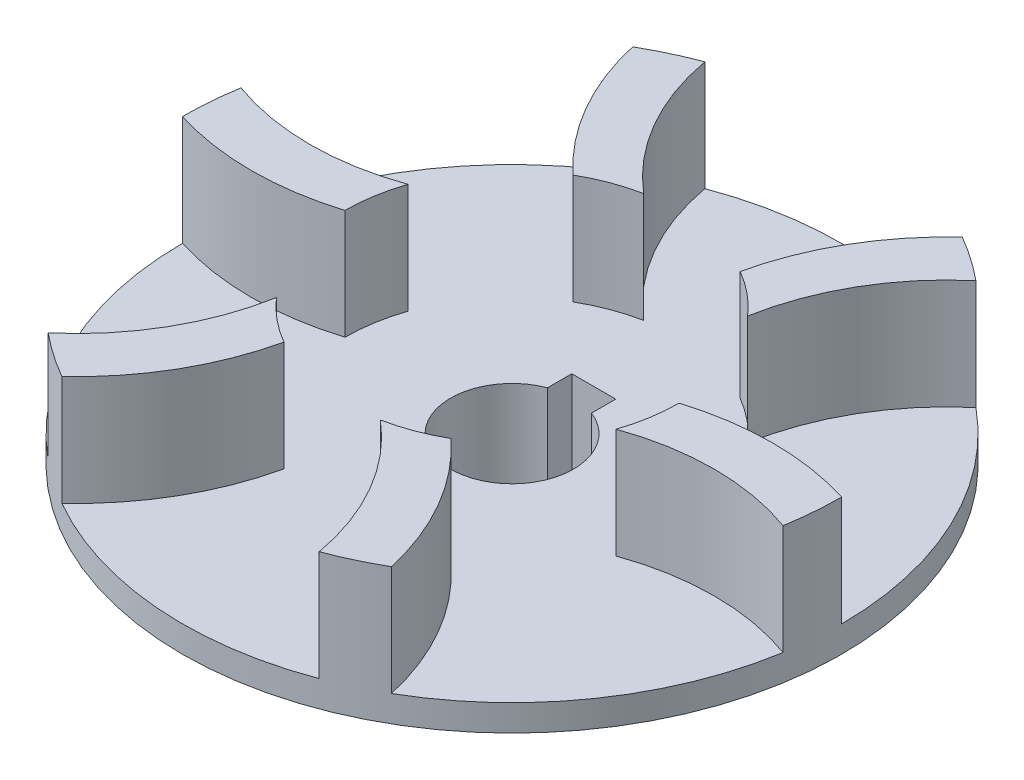
ISO-10303-21;
HEADER;
FILE_DESCRIPTION(('STEP AP214'),'2;1');
FILE_NAME('part.step','',(''),(''),'','','');
FILE_SCHEMA(('AUTOMOTIVE_DESIGN { 1 0 10303 214 1 1 1 1 }'));
ENDSEC;
DATA;
#1=APPLICATION_CONTEXT('core data for automotive mechanical design processes');
#2=APPLICATION_PROTOCOL_DEFINITION('international standard','automotive_design',2000,#1);
#3=PRODUCT_CONTEXT('',#1,'mechanical');
#4=PRODUCT('Part','Part','',(#3));
#5=PRODUCT_RELATED_PRODUCT_CATEGORY('part','',(#4));
#6=PRODUCT_DEFINITION_FORMATION('','',#4);
#7=PRODUCT_DEFINITION_CONTEXT('part definition',#1,'design');
#8=PRODUCT_DEFINITION('design','',#6,#7);
#9=PRODUCT_DEFINITION_SHAPE('','',#8);
#10=(LENGTH_UNIT() NAMED_UNIT(*) SI_UNIT(.MILLI.,.METRE.));
#11=(NAMED_UNIT(*) PLANE_ANGLE_UNIT() SI_UNIT($,.RADIAN.));
#12=(NAMED_UNIT(*) SI_UNIT($,.STERADIAN.) SOLID_ANGLE_UNIT());
#13=UNCERTAINTY_MEASURE_WITH_UNIT(LENGTH_MEASURE(1.E-05),#10,'distance_accuracy_value','');
#14=(GEOMETRIC_REPRESENTATION_CONTEXT(3) GLOBAL_UNCERTAINTY_ASSIGNED_CONTEXT((#13)) GLOBAL_UNIT_ASSIGNED_CONTEXT((#10,
#11,#12)) REPRESENTATION_CONTEXT('',''));
#15=CARTESIAN_POINT('',(0.,0.,0.));
#16=DIRECTION('',(0.,0.,1.));
#17=DIRECTION('',(1.,0.,0.));
#18=AXIS2_PLACEMENT_3D('',#15,#16,#17);
#19=CARTESIAN_POINT('',(0.,1.5,0.));
#20=DIRECTION('',(0.,-1.,0.));
#21=DIRECTION('',(0.,0.,-1.));
#22=AXIS2_PLACEMENT_3D('',#19,#20,#21);
#23=CYLINDRICAL_SURFACE('',#22,7.);
#24=DIRECTION('',(0.,-1.,0.));
#25=VECTOR('',#24,1.);
#26=CARTESIAN_POINT('',(2.5,1.5,-6.53834841531101));
#27=LINE('',#26,#25);
#28=CARTESIAN_POINT('',(2.5,1.5,-6.53834841531101));
#29=VERTEX_POINT('',#28);
#30=CARTESIAN_POINT('',(2.5,-17.5,-6.53834841531101));
#31=VERTEX_POINT('',#30);
#32=EDGE_CURVE('E238',#29,#31,#27,.T.);
#33=ORIENTED_EDGE('',*,*,#32,.T.);
#34=CARTESIAN_POINT('',(0.,-17.5,0.));
#35=DIRECTION('',(0.,-1.,0.));
#36=DIRECTION('',(0.,0.,-1.));
#37=AXIS2_PLACEMENT_3D('',#34,#35,#36);
#38=CIRCLE('',#37,7.);
#39=CARTESIAN_POINT('',(-2.5,-17.5,-6.53834841531101));
#40=VERTEX_POINT('',#39);
#41=EDGE_CURVE('E236',#40,#31,#38,.F.);
#42=ORIENTED_EDGE('',*,*,#41,.F.);
#43=DIRECTION('',(0.,-1.,0.));
#44=VECTOR('',#43,1.);
#45=CARTESIAN_POINT('',(-2.5,1.5,-6.53834841531101));
#46=LINE('',#45,#44);
#47=CARTESIAN_POINT('',(-2.5,1.5,-6.53834841531101));
#48=VERTEX_POINT('',#47);
#49=EDGE_CURVE('E221',#48,#40,#46,.T.);
#50=ORIENTED_EDGE('',*,*,#49,.F.);
#51=CARTESIAN_POINT('',(0.,1.5,0.));
#52=DIRECTION('',(0.,1.,0.));
#53=DIRECTION('',(0.,0.,1.));
#54=AXIS2_PLACEMENT_3D('',#51,#52,#53);
#55=CIRCLE('',#54,7.);
#56=EDGE_CURVE('E400',#48,#29,#55,.T.);
#57=ORIENTED_EDGE('',*,*,#56,.T.);
#58=EDGE_LOOP('',(#33,#42,#50,#57));
#59=FACE_BOUND('',#58,.T.);
#60=ADVANCED_FACE('F41',(#59),#23,.F.);
#61=CARTESIAN_POINT('',(-2.5,1.5,0.));
#62=DIRECTION('',(1.,0.,0.));
#63=DIRECTION('',(0.,0.,-1.));
#64=AXIS2_PLACEMENT_3D('',#61,#62,#63);
#65=PLANE('',#64);
#66=ORIENTED_EDGE('',*,*,#49,.T.);
#67=DIRECTION('',(0.,0.,1.));
#68=VECTOR('',#67,1.);
#69=CARTESIAN_POINT('',(-2.5,-17.5,0.));
#70=LINE('',#69,#68);
#71=CARTESIAN_POINT('',(-2.5,-17.5,-9.3));
#72=VERTEX_POINT('',#71);
#73=EDGE_CURVE('E230',#72,#40,#70,.T.);
#74=ORIENTED_EDGE('',*,*,#73,.F.);
#75=DIRECTION('',(0.,-1.,0.));
#76=VECTOR('',#75,1.);
#77=CARTESIAN_POINT('',(-2.5,1.5,-9.3));
#78=LINE('',#77,#76);
#79=CARTESIAN_POINT('',(-2.5,1.5,-9.3));
#80=VERTEX_POINT('',#79);
#81=EDGE_CURVE('E234',#80,#72,#78,.T.);
#82=ORIENTED_EDGE('',*,*,#81,.F.);
#83=DIRECTION('',(0.,0.,1.));
#84=VECTOR('',#83,1.);
#85=CARTESIAN_POINT('',(-2.5,1.5,0.));
#86=LINE('',#85,#84);
#87=EDGE_CURVE('E228',#80,#48,#86,.T.);
#88=ORIENTED_EDGE('',*,*,#87,.T.);
#89=EDGE_LOOP('',(#66,#74,#82,#88));
#90=FACE_BOUND('',#89,.T.);
#91=ADVANCED_FACE('F227',(#90),#65,.T.);
#92=CARTESIAN_POINT('',(0.,1.5,-9.3));
#93=DIRECTION('',(0.,0.,1.));
#94=DIRECTION('',(1.,0.,0.));
#95=AXIS2_PLACEMENT_3D('',#92,#93,#94);
#96=PLANE('',#95);
#97=ORIENTED_EDGE('',*,*,#81,.T.);
#98=DIRECTION('',(-1.,0.,0.));
#99=VECTOR('',#98,1.);
#100=CARTESIAN_POINT('',(0.,-17.5,-9.3));
#101=LINE('',#100,#99);
#102=CARTESIAN_POINT('',(2.5,-17.5,-9.3));
#103=VERTEX_POINT('',#102);
#104=EDGE_CURVE('E249',#103,#72,#101,.T.);
#105=ORIENTED_EDGE('',*,*,#104,.F.);
#106=DIRECTION('',(0.,-1.,0.));
#107=VECTOR('',#106,1.);
#108=CARTESIAN_POINT('',(2.5,1.5,-9.3));
#109=LINE('',#108,#107);
#110=CARTESIAN_POINT('',(2.5,1.5,-9.3));
#111=VERTEX_POINT('',#110);
#112=EDGE_CURVE('E415',#111,#103,#109,.T.);
#113=ORIENTED_EDGE('',*,*,#112,.F.);
#114=DIRECTION('',(-1.,0.,0.));
#115=VECTOR('',#114,1.);
#116=CARTESIAN_POINT('',(0.,1.5,-9.3));
#117=LINE('',#116,#115);
#118=EDGE_CURVE('E399',#111,#80,#117,.T.);
#119=ORIENTED_EDGE('',*,*,#118,.T.);
#120=EDGE_LOOP('',(#97,#105,#113,#119));
#121=FACE_BOUND('',#120,.T.);
#122=ADVANCED_FACE('F513',(#121),#96,.T.);
#123=CARTESIAN_POINT('',(2.5,1.5,0.));
#124=DIRECTION('',(1.,0.,0.));
#125=DIRECTION('',(0.,0.,-1.));
#126=AXIS2_PLACEMENT_3D('',#123,#124,#125);
#127=PLANE('',#126);
#128=ORIENTED_EDGE('',*,*,#112,.T.);
#129=DIRECTION('',(0.,0.,-1.));
#130=VECTOR('',#129,1.);
#131=CARTESIAN_POINT('',(2.5,-17.5,0.));
#132=LINE('',#131,#130);
#133=EDGE_CURVE('E241',#31,#103,#132,.T.);
#134=ORIENTED_EDGE('',*,*,#133,.F.);
#135=ORIENTED_EDGE('',*,*,#32,.F.);
#136=DIRECTION('',(0.,0.,1.));
#137=VECTOR('',#136,1.);
#138=CARTESIAN_POINT('',(2.5,1.5,0.));
#139=LINE('',#138,#137);
#140=EDGE_CURVE('E401',#111,#29,#139,.T.);
#141=ORIENTED_EDGE('',*,*,#140,.F.);
#142=EDGE_LOOP('',(#128,#134,#135,#141));
#143=FACE_BOUND('',#142,.T.);
#144=ADVANCED_FACE('F518',(#143),#127,.F.);
#145=CARTESIAN_POINT('',(0.,1.5,0.));
#146=DIRECTION('',(0.,-1.,0.));
#147=DIRECTION('',(0.,0.,-1.));
#148=AXIS2_PLACEMENT_3D('',#145,#146,#147);
#149=CYLINDRICAL_SURFACE('',#148,37.5);
#150=CARTESIAN_POINT('',(0.,1.5,0.));
#151=DIRECTION('',(0.,1.,0.));
#152=DIRECTION('',(0.,0.,1.));
#153=AXIS2_PLACEMENT_3D('',#150,#151,#152);
#154=CIRCLE('',#153,37.5);
#155=CARTESIAN_POINT('',(18.7500000000004,1.5,-32.4759526419162));
#156=VERTEX_POINT('',#155);
#157=CARTESIAN_POINT('',(-13.1678223706898,1.5,-35.1120841593597));
#158=VERTEX_POINT('',#157);
#159=EDGE_CURVE('E410',#156,#158,#154,.T.);
#160=ORIENTED_EDGE('',*,*,#159,.F.);
#161=DIRECTION('',(0.,-1.,0.));
#162=VECTOR('',#161,1.);
#163=CARTESIAN_POINT('',(18.7500000000004,14.,-32.4759526419162));
#164=LINE('',#163,#162);
#165=CARTESIAN_POINT('',(18.7500000000004,14.,-32.4759526419162));
#166=VERTEX_POINT('',#165);
#167=EDGE_CURVE('E261',#166,#156,#164,.T.);
#168=ORIENTED_EDGE('',*,*,#167,.F.);
#169=CARTESIAN_POINT('',(0.,14.,0.));
#170=DIRECTION('',(0.,1.,0.));
#171=DIRECTION('',(0.,0.,1.));
#172=AXIS2_PLACEMENT_3D('',#169,#170,#171);
#173=CIRCLE('',#172,37.5);
#174=CARTESIAN_POINT('',(23.8240456764779,14.,-28.9597107652182));
#175=VERTEX_POINT('',#174);
#176=EDGE_CURVE('E277',#175,#166,#173,.T.);
#177=ORIENTED_EDGE('',*,*,#176,.F.);
#178=DIRECTION('',(0.,-1.,0.));
#179=VECTOR('',#178,1.);
#180=CARTESIAN_POINT('',(23.8240456764779,14.,-28.9597107652182));
#181=LINE('',#180,#179);
#182=CARTESIAN_POINT('',(23.8240456764779,1.5,-28.9597107652182));
#183=VERTEX_POINT('',#182);
#184=EDGE_CURVE('E256',#175,#183,#181,.T.);
#185=ORIENTED_EDGE('',*,*,#184,.T.);
#186=CARTESIAN_POINT('',(37.5,1.5,0.));
#187=VERTEX_POINT('',#186);
#188=EDGE_CURVE('E407',#187,#183,#154,.T.);
#189=ORIENTED_EDGE('',*,*,#188,.F.);
#190=DIRECTION('',(0.,-1.,0.));
#191=VECTOR('',#190,1.);
#192=CARTESIAN_POINT('',(37.5,14.,0.));
#193=LINE('',#192,#191);
#194=CARTESIAN_POINT('',(37.5,14.,0.));
#195=VERTEX_POINT('',#194);
#196=EDGE_CURVE('E388',#195,#187,#193,.T.);
#197=ORIENTED_EDGE('',*,*,#196,.F.);
#198=CARTESIAN_POINT('',(0.,14.,0.));
#199=DIRECTION('',(0.,1.,0.));
#200=DIRECTION('',(0.,0.,1.));
#201=AXIS2_PLACEMENT_3D('',#198,#199,#200);
#202=CIRCLE('',#201,37.5);
#203=CARTESIAN_POINT('',(36.9918680471677,14.,6.15237339414113));
#204=VERTEX_POINT('',#203);
#205=EDGE_CURVE('E376',#204,#195,#202,.T.);
#206=ORIENTED_EDGE('',*,*,#205,.F.);
#207=DIRECTION('',(0.,-1.,0.));
#208=VECTOR('',#207,1.);
#209=CARTESIAN_POINT('',(36.9918680471677,14.,6.15237339414113));
#210=LINE('',#209,#208);
#211=CARTESIAN_POINT('',(36.9918680471677,1.5,6.15237339414113));
#212=VERTEX_POINT('',#211);
#213=EDGE_CURVE('E395',#204,#212,#210,.T.);
#214=ORIENTED_EDGE('',*,*,#213,.T.);
#215=CARTESIAN_POINT('',(18.7499999999999,1.5,32.4759526419165));
#216=VERTEX_POINT('',#215);
#217=EDGE_CURVE('E403',#216,#212,#154,.T.);
#218=ORIENTED_EDGE('',*,*,#217,.F.);
#219=DIRECTION('',(0.,-1.,0.));
#220=VECTOR('',#219,1.);
#221=CARTESIAN_POINT('',(18.7499999999999,14.,32.4759526419165));
#222=LINE('',#221,#220);
#223=CARTESIAN_POINT('',(18.7499999999999,14.,32.4759526419165));
#224=VERTEX_POINT('',#223);
#225=EDGE_CURVE('E355',#224,#216,#222,.T.);
#226=ORIENTED_EDGE('',*,*,#225,.F.);
#227=CARTESIAN_POINT('',(0.,14.,0.));
#228=DIRECTION('',(0.,1.,0.));
#229=DIRECTION('',(0.,0.,1.));
#230=AXIS2_PLACEMENT_3D('',#227,#228,#229);
#231=CIRCLE('',#230,37.5);
#232=CARTESIAN_POINT('',(13.16782237069,14.,35.1120841593597));
#233=VERTEX_POINT('',#232);
#234=EDGE_CURVE('E366',#233,#224,#231,.T.);
#235=ORIENTED_EDGE('',*,*,#234,.F.);
#236=DIRECTION('',(0.,-1.,0.));
#237=VECTOR('',#236,1.);
#238=CARTESIAN_POINT('',(13.16782237069,14.,35.1120841593597));
#239=LINE('',#238,#237);
#240=CARTESIAN_POINT('',(13.16782237069,1.5,35.1120841593597));
#241=VERTEX_POINT('',#240);
#242=EDGE_CURVE('E348',#233,#241,#239,.T.);
#243=ORIENTED_EDGE('',*,*,#242,.T.);
#244=CARTESIAN_POINT('',(-18.7500000000001,1.5,32.4759526419164));
#245=VERTEX_POINT('',#244);
#246=EDGE_CURVE('E477',#245,#241,#154,.T.);
#247=ORIENTED_EDGE('',*,*,#246,.F.);
#248=DIRECTION('',(0.,-1.,0.));
#249=VECTOR('',#248,1.);
#250=CARTESIAN_POINT('',(-18.7500000000002,14.,32.4759526419164));
#251=LINE('',#250,#249);
#252=CARTESIAN_POINT('',(-18.7500000000002,14.,32.4759526419164));
#253=VERTEX_POINT('',#252);
#254=EDGE_CURVE('E329',#253,#245,#251,.T.);
#255=ORIENTED_EDGE('',*,*,#254,.F.);
#256=CARTESIAN_POINT('',(0.,14.,0.));
#257=DIRECTION('',(0.,1.,0.));
#258=DIRECTION('',(0.,0.,1.));
#259=AXIS2_PLACEMENT_3D('',#256,#257,#258);
#260=CIRCLE('',#259,37.5);
#261=CARTESIAN_POINT('',(-23.8240456764777,14.,28.9597107652184));
#262=VERTEX_POINT('',#261);
#263=EDGE_CURVE('E344',#262,#253,#260,.T.);
#264=ORIENTED_EDGE('',*,*,#263,.F.);
#265=DIRECTION('',(0.,-1.,0.));
#266=VECTOR('',#265,1.);
#267=CARTESIAN_POINT('',(-23.8240456764777,14.,28.9597107652184));
#268=LINE('',#267,#266);
#269=CARTESIAN_POINT('',(-23.8240456764777,1.5,28.9597107652184));
#270=VERTEX_POINT('',#269);
#271=EDGE_CURVE('E330',#262,#270,#268,.T.);
#272=ORIENTED_EDGE('',*,*,#271,.T.);
#273=CARTESIAN_POINT('',(-37.5,1.5,-2.63677968348475E-13));
#274=VERTEX_POINT('',#273);
#275=EDGE_CURVE('E480',#274,#270,#154,.T.);
#276=ORIENTED_EDGE('',*,*,#275,.F.);
#277=DIRECTION('',(0.,-1.,0.));
#278=VECTOR('',#277,1.);
#279=CARTESIAN_POINT('',(-37.5,14.,-2.63677968348475E-13));
#280=LINE('',#279,#278);
#281=CARTESIAN_POINT('',(-37.5,14.,-2.63677968348475E-13));
#282=VERTEX_POINT('',#281);
#283=EDGE_CURVE('E307',#282,#274,#280,.T.);
#284=ORIENTED_EDGE('',*,*,#283,.F.);
#285=CARTESIAN_POINT('',(0.,14.,0.));
#286=DIRECTION('',(0.,1.,0.));
#287=DIRECTION('',(0.,0.,1.));
#288=AXIS2_PLACEMENT_3D('',#285,#286,#287);
#289=CIRCLE('',#288,37.5);
#290=CARTESIAN_POINT('',(-36.9918680471676,14.,-6.15237339414141));
#291=VERTEX_POINT('',#290);
#292=EDGE_CURVE('E325',#291,#282,#289,.T.);
#293=ORIENTED_EDGE('',*,*,#292,.F.);
#294=DIRECTION('',(0.,-1.,0.));
#295=VECTOR('',#294,1.);
#296=CARTESIAN_POINT('',(-36.9918680471676,14.,-6.15237339414141));
#297=LINE('',#296,#295);
#298=CARTESIAN_POINT('',(-36.9918680471676,1.5,-6.15237339414141));
#299=VERTEX_POINT('',#298);
#300=EDGE_CURVE('E302',#291,#299,#297,.T.);
#301=ORIENTED_EDGE('',*,*,#300,.T.);
#302=CARTESIAN_POINT('',(-18.7499999999997,1.5,-32.4759526419166));
#303=VERTEX_POINT('',#302);
#304=EDGE_CURVE('E478',#303,#299,#154,.T.);
#305=ORIENTED_EDGE('',*,*,#304,.F.);
#306=DIRECTION('',(0.,-1.,0.));
#307=VECTOR('',#306,1.);
#308=CARTESIAN_POINT('',(-18.7499999999997,14.,-32.4759526419166));
#309=LINE('',#308,#307);
#310=CARTESIAN_POINT('',(-18.7499999999997,14.,-32.4759526419166));
#311=VERTEX_POINT('',#310);
#312=EDGE_CURVE('E281',#311,#303,#309,.T.);
#313=ORIENTED_EDGE('',*,*,#312,.F.);
#314=CARTESIAN_POINT('',(0.,14.,0.));
#315=DIRECTION('',(0.,1.,0.));
#316=DIRECTION('',(0.,0.,1.));
#317=AXIS2_PLACEMENT_3D('',#314,#315,#316);
#318=CIRCLE('',#317,37.5);
#319=CARTESIAN_POINT('',(-13.1678223706898,14.,-35.1120841593597));
#320=VERTEX_POINT('',#319);
#321=EDGE_CURVE('E296',#320,#311,#318,.T.);
#322=ORIENTED_EDGE('',*,*,#321,.F.);
#323=DIRECTION('',(0.,-1.,0.));
#324=VECTOR('',#323,1.);
#325=CARTESIAN_POINT('',(-13.1678223706898,14.,-35.1120841593597));
#326=LINE('',#325,#324);
#327=EDGE_CURVE('E282',#320,#158,#326,.T.);
#328=ORIENTED_EDGE('',*,*,#327,.T.);
#329=EDGE_LOOP('',(#160,#168,#177,#185,#189,#197,#206,#214,#218,#226,#235,#243,#247,#255,#264,
#272,#276,#284,#293,#301,#305,#313,#322,#328));
#330=FACE_BOUND('',#329,.T.);
#331=CARTESIAN_POINT('',(0.,-1.5,0.));
#332=DIRECTION('',(0.,1.,0.));
#333=DIRECTION('',(0.,0.,1.));
#334=AXIS2_PLACEMENT_3D('',#331,#332,#333);
#335=CIRCLE('',#334,37.5);
#336=CARTESIAN_POINT('',(0.,-1.5,37.5));
#337=VERTEX_POINT('',#336);
#338=EDGE_CURVE('E396',#337,#337,#335,.T.);
#339=ORIENTED_EDGE('',*,*,#338,.T.);
#340=EDGE_LOOP('',(#339));
#341=FACE_BOUND('',#340,.T.);
#342=ADVANCED_FACE('F472',(#330,#341),#149,.T.);
#343=CARTESIAN_POINT('',(0.,1.5,0.));
#344=DIRECTION('',(0.,1.,0.));
#345=DIRECTION('',(0.,0.,1.));
#346=AXIS2_PLACEMENT_3D('',#343,#344,#345);
#347=PLANE('',#346);
#348=ORIENTED_EDGE('',*,*,#56,.F.);
#349=ORIENTED_EDGE('',*,*,#87,.F.);
#350=ORIENTED_EDGE('',*,*,#118,.F.);
#351=ORIENTED_EDGE('',*,*,#140,.T.);
#352=EDGE_LOOP('',(#348,#349,#350,#351));
#353=FACE_BOUND('',#352,.T.);
#354=ORIENTED_EDGE('',*,*,#188,.T.);
#355=CARTESIAN_POINT('',(41.8753460220925,1.5,-7.55525898918773));
#356=DIRECTION('',(0.,1.,0.));
#357=DIRECTION('',(0.,0.,1.));
#358=AXIS2_PLACEMENT_3D('',#355,#356,#357);
#359=CIRCLE('',#358,28.);
#360=CARTESIAN_POINT('',(14.3143410715171,1.5,-12.4939841399082));
#361=VERTEX_POINT('',#360);
#362=EDGE_CURVE('E47',#183,#361,#359,.T.);
#363=ORIENTED_EDGE('',*,*,#362,.T.);
#364=CARTESIAN_POINT('',(0.,1.5,0.));
#365=DIRECTION('',(0.,1.,0.));
#366=DIRECTION('',(0.,0.,1.));
#367=AXIS2_PLACEMENT_3D('',#364,#365,#366);
#368=CIRCLE('',#367,19.);
#369=CARTESIAN_POINT('',(9.50000000000019,1.5,-16.4544826719042));
#370=VERTEX_POINT('',#369);
#371=EDGE_CURVE('E57',#370,#361,#368,.F.);
#372=ORIENTED_EDGE('',*,*,#371,.F.);
#373=CARTESIAN_POINT('',(39.7487804587849,1.5,-9.67132111137468));
#374=DIRECTION('',(0.,1.,0.));
#375=DIRECTION('',(0.,0.,1.));
#376=AXIS2_PLACEMENT_3D('',#373,#374,#375);
#377=CIRCLE('',#376,31.);
#378=EDGE_CURVE('E58',#156,#370,#377,.T.);
#379=ORIENTED_EDGE('',*,*,#378,.F.);
#380=ORIENTED_EDGE('',*,*,#159,.T.);
#381=CARTESIAN_POINT('',(14.3946267942388,1.5,-40.0427429419896));
#382=DIRECTION('',(0.,1.,0.));
#383=DIRECTION('',(0.,0.,1.));
#384=AXIS2_PLACEMENT_3D('',#381,#382,#383);
#385=CIRCLE('',#384,28.);
#386=CARTESIAN_POINT('',(-3.66293712388191,1.5,-18.6435750763229));
#387=VERTEX_POINT('',#386);
#388=EDGE_CURVE('E455',#158,#387,#385,.T.);
#389=ORIENTED_EDGE('',*,*,#388,.T.);
#390=CARTESIAN_POINT('',(0.,1.5,0.));
#391=DIRECTION('',(0.,1.,0.));
#392=DIRECTION('',(0.,0.,1.));
#393=AXIS2_PLACEMENT_3D('',#390,#391,#392);
#394=CIRCLE('',#393,19.);
#395=CARTESIAN_POINT('',(-9.49999999999985,1.5,-16.4544826719044));
#396=VERTEX_POINT('',#395);
#397=EDGE_CURVE('E447',#396,#387,#394,.F.);
#398=ORIENTED_EDGE('',*,*,#397,.F.);
#399=CARTESIAN_POINT('',(11.4987804587851,1.5,-39.2591142024455));
#400=DIRECTION('',(0.,1.,0.));
#401=DIRECTION('',(0.,0.,1.));
#402=AXIS2_PLACEMENT_3D('',#399,#400,#401);
#403=CIRCLE('',#402,31.);
#404=EDGE_CURVE('E446',#303,#396,#403,.T.);
#405=ORIENTED_EDGE('',*,*,#404,.F.);
#406=ORIENTED_EDGE('',*,*,#304,.T.);
#407=CARTESIAN_POINT('',(-27.4807192278537,1.5,-32.4874839528017));
#408=DIRECTION('',(0.,1.,0.));
#409=DIRECTION('',(0.,0.,1.));
#410=AXIS2_PLACEMENT_3D('',#407,#408,#409);
#411=CIRCLE('',#410,28.);
#412=CARTESIAN_POINT('',(-17.977278195399,1.5,-6.14959093641456));
#413=VERTEX_POINT('',#412);
#414=EDGE_CURVE('E441',#299,#413,#411,.T.);
#415=ORIENTED_EDGE('',*,*,#414,.T.);
#416=CARTESIAN_POINT('',(0.,1.5,0.));
#417=DIRECTION('',(0.,1.,0.));
#418=DIRECTION('',(0.,0.,1.));
#419=AXIS2_PLACEMENT_3D('',#416,#417,#418);
#420=CIRCLE('',#419,19.);
#421=CARTESIAN_POINT('',(-19.,1.5,-1.38493363171989E-13));
#422=VERTEX_POINT('',#421);
#423=EDGE_CURVE('E437',#422,#413,#420,.F.);
#424=ORIENTED_EDGE('',*,*,#423,.F.);
#425=CARTESIAN_POINT('',(-28.2499999999998,1.5,-29.5877930910707));
#426=DIRECTION('',(0.,1.,0.));
#427=DIRECTION('',(0.,0.,1.));
#428=AXIS2_PLACEMENT_3D('',#425,#426,#427);
#429=CIRCLE('',#428,31.);
#430=EDGE_CURVE('E442',#274,#422,#429,.T.);
#431=ORIENTED_EDGE('',*,*,#430,.F.);
#432=ORIENTED_EDGE('',*,*,#275,.T.);
#433=CARTESIAN_POINT('',(-41.8753460220924,1.5,7.55525898918802));
#434=DIRECTION('',(0.,1.,0.));
#435=DIRECTION('',(0.,0.,1.));
#436=AXIS2_PLACEMENT_3D('',#433,#434,#435);
#437=CIRCLE('',#436,28.);
#438=CARTESIAN_POINT('',(-14.314341071517,1.5,12.4939841399083));
#439=VERTEX_POINT('',#438);
#440=EDGE_CURVE('E436',#270,#439,#437,.T.);
#441=ORIENTED_EDGE('',*,*,#440,.T.);
#442=CARTESIAN_POINT('',(0.,1.5,0.));
#443=DIRECTION('',(0.,1.,0.));
#444=DIRECTION('',(0.,0.,1.));
#445=AXIS2_PLACEMENT_3D('',#442,#443,#444);
#446=CIRCLE('',#445,19.);
#447=CARTESIAN_POINT('',(-9.50000000000008,1.5,16.4544826719043));
#448=VERTEX_POINT('',#447);
#449=EDGE_CURVE('E429',#448,#439,#446,.F.);
#450=ORIENTED_EDGE('',*,*,#449,.F.);
#451=CARTESIAN_POINT('',(-39.7487804587848,1.5,9.67132111137496));
#452=DIRECTION('',(0.,1.,0.));
#453=DIRECTION('',(0.,0.,1.));
#454=AXIS2_PLACEMENT_3D('',#451,#452,#453);
#455=CIRCLE('',#454,31.);
#456=EDGE_CURVE('E433',#245,#448,#455,.T.);
#457=ORIENTED_EDGE('',*,*,#456,.F.);
#458=ORIENTED_EDGE('',*,*,#246,.T.);
#459=CARTESIAN_POINT('',(-14.3946267942386,1.5,40.0427429419897));
#460=DIRECTION('',(0.,1.,0.));
#461=DIRECTION('',(0.,0.,1.));
#462=AXIS2_PLACEMENT_3D('',#459,#460,#461);
#463=CIRCLE('',#462,28.);
#464=CARTESIAN_POINT('',(3.66293712388204,1.5,18.6435750763229));
#465=VERTEX_POINT('',#464);
#466=EDGE_CURVE('E428',#241,#465,#463,.T.);
#467=ORIENTED_EDGE('',*,*,#466,.T.);
#468=CARTESIAN_POINT('',(0.,1.5,0.));
#469=DIRECTION('',(0.,1.,0.));
#470=DIRECTION('',(0.,0.,1.));
#471=AXIS2_PLACEMENT_3D('',#468,#469,#470);
#472=CIRCLE('',#471,19.);
#473=CARTESIAN_POINT('',(9.49999999999996,1.5,16.4544826719044));
#474=VERTEX_POINT('',#473);
#475=EDGE_CURVE('E425',#474,#465,#472,.F.);
#476=ORIENTED_EDGE('',*,*,#475,.F.);
#477=CARTESIAN_POINT('',(-11.4987804587849,1.5,39.2591142024456));
#478=DIRECTION('',(0.,1.,0.));
#479=DIRECTION('',(0.,0.,1.));
#480=AXIS2_PLACEMENT_3D('',#477,#478,#479);
#481=CIRCLE('',#480,31.);
#482=EDGE_CURVE('E422',#216,#474,#481,.T.);
#483=ORIENTED_EDGE('',*,*,#482,.F.);
#484=ORIENTED_EDGE('',*,*,#217,.T.);
#485=CARTESIAN_POINT('',(27.4807192278539,1.5,32.4874839528015));
#486=DIRECTION('',(0.,1.,0.));
#487=DIRECTION('',(0.,0.,1.));
#488=AXIS2_PLACEMENT_3D('',#485,#486,#487);
#489=CIRCLE('',#488,28.);
#490=CARTESIAN_POINT('',(17.977278195399,1.5,6.14959093641443));
#491=VERTEX_POINT('',#490);
#492=EDGE_CURVE('E419',#212,#491,#489,.T.);
#493=ORIENTED_EDGE('',*,*,#492,.T.);
#494=CARTESIAN_POINT('',(0.,1.5,0.));
#495=DIRECTION('',(0.,1.,0.));
#496=DIRECTION('',(0.,0.,1.));
#497=AXIS2_PLACEMENT_3D('',#494,#495,#496);
#498=CIRCLE('',#497,19.);
#499=CARTESIAN_POINT('',(19.,1.5,0.));
#500=VERTEX_POINT('',#499);
#501=EDGE_CURVE('E232',#500,#491,#498,.F.);
#502=ORIENTED_EDGE('',*,*,#501,.F.);
#503=CARTESIAN_POINT('',(28.25,1.5,29.5877930910705));
#504=DIRECTION('',(0.,1.,0.));
#505=DIRECTION('',(0.,0.,1.));
#506=AXIS2_PLACEMENT_3D('',#503,#504,#505);
#507=CIRCLE('',#506,31.);
#508=EDGE_CURVE('E417',#187,#500,#507,.T.);
#509=ORIENTED_EDGE('',*,*,#508,.F.);
#510=EDGE_LOOP('',(#354,#363,#372,#379,#380,#389,#398,#405,#406,#415,#424,#431,#432,#441,#450,
#457,#458,#467,#476,#483,#484,#493,#502,#509));
#511=FACE_BOUND('',#510,.T.);
#512=ADVANCED_FACE('F457',(#353,#511),#347,.T.);
#513=CARTESIAN_POINT('',(0.,-1.5,0.));
#514=DIRECTION('',(0.,1.,0.));
#515=DIRECTION('',(0.,0.,1.));
#516=AXIS2_PLACEMENT_3D('',#513,#514,#515);
#517=PLANE('',#516);
#518=CARTESIAN_POINT('',(0.,-1.5,0.));
#519=DIRECTION('',(0.,1.,0.));
#520=DIRECTION('',(0.,0.,1.));
#521=AXIS2_PLACEMENT_3D('',#518,#519,#520);
#522=CIRCLE('',#521,28.5);
#523=CARTESIAN_POINT('',(0.,-1.5,28.5));
#524=VERTEX_POINT('',#523);
#525=EDGE_CURVE('E11',#524,#524,#522,.T.);
#526=ORIENTED_EDGE('',*,*,#525,.T.);
#527=EDGE_LOOP('',(#526));
#528=FACE_BOUND('',#527,.T.);
#529=ORIENTED_EDGE('',*,*,#338,.F.);
#530=EDGE_LOOP('',(#529));
#531=FACE_BOUND('',#530,.T.);
#532=ADVANCED_FACE('F508',(#528,#531),#517,.F.);
#533=CARTESIAN_POINT('',(27.4807192278539,14.,32.4874839528015));
#534=DIRECTION('',(0.,-1.,0.));
#535=DIRECTION('',(0.,0.,-1.));
#536=AXIS2_PLACEMENT_3D('',#533,#534,#535);
#537=CYLINDRICAL_SURFACE('',#536,28.);
#538=ORIENTED_EDGE('',*,*,#492,.F.);
#539=ORIENTED_EDGE('',*,*,#213,.F.);
#540=CARTESIAN_POINT('',(27.4807192278539,14.,32.4874839528015));
#541=DIRECTION('',(0.,-1.,0.));
#542=DIRECTION('',(0.,0.,-1.));
#543=AXIS2_PLACEMENT_3D('',#540,#541,#542);
#544=CIRCLE('',#543,28.);
#545=CARTESIAN_POINT('',(17.977278195399,14.,6.14959093641443));
#546=VERTEX_POINT('',#545);
#547=EDGE_CURVE('E373',#546,#204,#544,.T.);
#548=ORIENTED_EDGE('',*,*,#547,.F.);
#549=DIRECTION('',(0.,-1.,0.));
#550=VECTOR('',#549,1.);
#551=CARTESIAN_POINT('',(17.977278195399,14.,6.14959093641443));
#552=LINE('',#551,#550);
#553=EDGE_CURVE('E383',#546,#491,#552,.T.);
#554=ORIENTED_EDGE('',*,*,#553,.T.);
#555=EDGE_LOOP('',(#538,#539,#548,#554));
#556=FACE_BOUND('',#555,.T.);
#557=ADVANCED_FACE('F489',(#556),#537,.F.);
#558=CARTESIAN_POINT('',(28.25,14.,29.5877930910705));
#559=DIRECTION('',(0.,-1.,0.));
#560=DIRECTION('',(0.,0.,-1.));
#561=AXIS2_PLACEMENT_3D('',#558,#559,#560);
#562=CYLINDRICAL_SURFACE('',#561,31.);
#563=ORIENTED_EDGE('',*,*,#196,.T.);
#564=ORIENTED_EDGE('',*,*,#508,.T.);
#565=DIRECTION('',(0.,-1.,0.));
#566=VECTOR('',#565,1.);
#567=CARTESIAN_POINT('',(19.,14.,0.));
#568=LINE('',#567,#566);
#569=CARTESIAN_POINT('',(19.,14.,0.));
#570=VERTEX_POINT('',#569);
#571=EDGE_CURVE('E390',#570,#500,#568,.T.);
#572=ORIENTED_EDGE('',*,*,#571,.F.);
#573=CARTESIAN_POINT('',(28.25,14.,29.5877930910705));
#574=DIRECTION('',(0.,-1.,0.));
#575=DIRECTION('',(0.,0.,-1.));
#576=AXIS2_PLACEMENT_3D('',#573,#574,#575);
#577=CIRCLE('',#576,31.);
#578=EDGE_CURVE('E378',#570,#195,#577,.T.);
#579=ORIENTED_EDGE('',*,*,#578,.T.);
#580=EDGE_LOOP('',(#563,#564,#572,#579));
#581=FACE_BOUND('',#580,.T.);
#582=ADVANCED_FACE('F498',(#581),#562,.T.);
#583=CARTESIAN_POINT('',(0.,14.,0.));
#584=DIRECTION('',(0.,-1.,0.));
#585=DIRECTION('',(0.,0.,-1.));
#586=AXIS2_PLACEMENT_3D('',#583,#584,#585);
#587=CYLINDRICAL_SURFACE('',#586,19.);
#588=ORIENTED_EDGE('',*,*,#571,.T.);
#589=ORIENTED_EDGE('',*,*,#501,.T.);
#590=ORIENTED_EDGE('',*,*,#553,.F.);
#591=CARTESIAN_POINT('',(0.,14.,0.));
#592=DIRECTION('',(0.,1.,0.));
#593=DIRECTION('',(0.,0.,1.));
#594=AXIS2_PLACEMENT_3D('',#591,#592,#593);
#595=CIRCLE('',#594,19.);
#596=EDGE_CURVE('E381',#546,#570,#595,.T.);
#597=ORIENTED_EDGE('',*,*,#596,.T.);
#598=EDGE_LOOP('',(#588,#589,#590,#597));
#599=FACE_BOUND('',#598,.T.);
#600=ADVANCED_FACE('F499',(#599),#587,.F.);
#601=CARTESIAN_POINT('',(13.740359613927,14.,16.2437419764008));
#602=DIRECTION('',(0.,-1.,0.));
#603=DIRECTION('',(0.,0.,-1.));
#604=AXIS2_PLACEMENT_3D('',#601,#602,#603);
#605=PLANE('',#604);
#606=ORIENTED_EDGE('',*,*,#547,.T.);
#607=ORIENTED_EDGE('',*,*,#205,.T.);
#608=ORIENTED_EDGE('',*,*,#578,.F.);
#609=ORIENTED_EDGE('',*,*,#596,.F.);
#610=EDGE_LOOP('',(#606,#607,#608,#609));
#611=FACE_BOUND('',#610,.T.);
#612=ADVANCED_FACE('F497',(#611),#605,.F.);
#613=CARTESIAN_POINT('',(-14.3946267942386,14.,40.0427429419897));
#614=DIRECTION('',(0.,-1.,0.));
#615=DIRECTION('',(0.,0.,-1.));
#616=AXIS2_PLACEMENT_3D('',#613,#614,#615);
#617=CYLINDRICAL_SURFACE('',#616,28.);
#618=ORIENTED_EDGE('',*,*,#466,.F.);
#619=ORIENTED_EDGE('',*,*,#242,.F.);
#620=CARTESIAN_POINT('',(-14.3946267942386,14.,40.0427429419897));
#621=DIRECTION('',(0.,-1.,0.));
#622=DIRECTION('',(0.,0.,-1.));
#623=AXIS2_PLACEMENT_3D('',#620,#621,#622);
#624=CIRCLE('',#623,28.);
#625=CARTESIAN_POINT('',(3.66293712388204,14.,18.6435750763229));
#626=VERTEX_POINT('',#625);
#627=EDGE_CURVE('E367',#626,#233,#624,.T.);
#628=ORIENTED_EDGE('',*,*,#627,.F.);
#629=DIRECTION('',(0.,-1.,0.));
#630=VECTOR('',#629,1.);
#631=CARTESIAN_POINT('',(3.66293712388204,14.,18.6435750763229));
#632=LINE('',#631,#630);
#633=EDGE_CURVE('E357',#626,#465,#632,.T.);
#634=ORIENTED_EDGE('',*,*,#633,.T.);
#635=EDGE_LOOP('',(#618,#619,#628,#634));
#636=FACE_BOUND('',#635,.T.);
#637=ADVANCED_FACE('F569',(#636),#617,.F.);
#638=CARTESIAN_POINT('',(-11.4987804587849,14.,39.2591142024456));
#639=DIRECTION('',(0.,-1.,0.));
#640=DIRECTION('',(0.,0.,-1.));
#641=AXIS2_PLACEMENT_3D('',#638,#639,#640);
#642=CYLINDRICAL_SURFACE('',#641,31.);
#643=ORIENTED_EDGE('',*,*,#225,.T.);
#644=ORIENTED_EDGE('',*,*,#482,.T.);
#645=DIRECTION('',(0.,-1.,0.));
#646=VECTOR('',#645,1.);
#647=CARTESIAN_POINT('',(9.49999999999996,14.,16.4544826719044));
#648=LINE('',#647,#646);
#649=CARTESIAN_POINT('',(9.49999999999996,14.,16.4544826719044));
#650=VERTEX_POINT('',#649);
#651=EDGE_CURVE('E356',#650,#474,#648,.T.);
#652=ORIENTED_EDGE('',*,*,#651,.F.);
#653=CARTESIAN_POINT('',(-11.4987804587849,14.,39.2591142024456));
#654=DIRECTION('',(0.,-1.,0.));
#655=DIRECTION('',(0.,0.,-1.));
#656=AXIS2_PLACEMENT_3D('',#653,#654,#655);
#657=CIRCLE('',#656,31.);
#658=EDGE_CURVE('E364',#650,#224,#657,.T.);
#659=ORIENTED_EDGE('',*,*,#658,.T.);
#660=EDGE_LOOP('',(#643,#644,#652,#659));
#661=FACE_BOUND('',#660,.T.);
#662=ADVANCED_FACE('F578',(#661),#642,.T.);
#663=CARTESIAN_POINT('',(0.,14.,0.));
#664=DIRECTION('',(0.,-1.,0.));
#665=DIRECTION('',(0.,0.,-1.));
#666=AXIS2_PLACEMENT_3D('',#663,#664,#665);
#667=CYLINDRICAL_SURFACE('',#666,19.);
#668=ORIENTED_EDGE('',*,*,#651,.T.);
#669=ORIENTED_EDGE('',*,*,#475,.T.);
#670=ORIENTED_EDGE('',*,*,#633,.F.);
#671=CARTESIAN_POINT('',(0.,14.,0.));
#672=DIRECTION('',(0.,1.,0.));
#673=DIRECTION('',(0.,0.,1.));
#674=AXIS2_PLACEMENT_3D('',#671,#672,#673);
#675=CIRCLE('',#674,19.);
#676=EDGE_CURVE('E362',#626,#650,#675,.T.);
#677=ORIENTED_EDGE('',*,*,#676,.T.);
#678=EDGE_LOOP('',(#668,#669,#670,#677));
#679=FACE_BOUND('',#678,.T.);
#680=ADVANCED_FACE('F586',(#679),#667,.F.);
#681=CARTESIAN_POINT('',(-7.19731339711928,14.,20.0213714709949));
#682=DIRECTION('',(0.,-1.,0.));
#683=DIRECTION('',(0.,0.,-1.));
#684=AXIS2_PLACEMENT_3D('',#681,#682,#683);
#685=PLANE('',#684);
#686=ORIENTED_EDGE('',*,*,#627,.T.);
#687=ORIENTED_EDGE('',*,*,#234,.T.);
#688=ORIENTED_EDGE('',*,*,#658,.F.);
#689=ORIENTED_EDGE('',*,*,#676,.F.);
#690=EDGE_LOOP('',(#686,#687,#688,#689));
#691=FACE_BOUND('',#690,.T.);
#692=ADVANCED_FACE('F598',(#691),#685,.F.);
#693=CARTESIAN_POINT('',(-41.8753460220924,14.,7.55525898918802));
#694=DIRECTION('',(0.,-1.,0.));
#695=DIRECTION('',(0.,0.,-1.));
#696=AXIS2_PLACEMENT_3D('',#693,#694,#695);
#697=CYLINDRICAL_SURFACE('',#696,28.);
#698=ORIENTED_EDGE('',*,*,#440,.F.);
#699=ORIENTED_EDGE('',*,*,#271,.F.);
#700=CARTESIAN_POINT('',(-41.8753460220924,14.,7.55525898918802));
#701=DIRECTION('',(0.,-1.,0.));
#702=DIRECTION('',(0.,0.,-1.));
#703=AXIS2_PLACEMENT_3D('',#700,#701,#702);
#704=CIRCLE('',#703,28.);
#705=CARTESIAN_POINT('',(-14.314341071517,14.,12.4939841399083));
#706=VERTEX_POINT('',#705);
#707=EDGE_CURVE('E350',#706,#262,#704,.T.);
#708=ORIENTED_EDGE('',*,*,#707,.F.);
#709=DIRECTION('',(0.,-1.,0.));
#710=VECTOR('',#709,1.);
#711=CARTESIAN_POINT('',(-14.314341071517,14.,12.4939841399083));
#712=LINE('',#711,#710);
#713=EDGE_CURVE('E337',#706,#439,#712,.T.);
#714=ORIENTED_EDGE('',*,*,#713,.T.);
#715=EDGE_LOOP('',(#698,#699,#708,#714));
#716=FACE_BOUND('',#715,.T.);
#717=ADVANCED_FACE('F609',(#716),#697,.F.);
#718=CARTESIAN_POINT('',(-39.7487804587848,14.,9.67132111137496));
#719=DIRECTION('',(0.,-1.,0.));
#720=DIRECTION('',(0.,0.,-1.));
#721=AXIS2_PLACEMENT_3D('',#718,#719,#720);
#722=CYLINDRICAL_SURFACE('',#721,31.);
#723=ORIENTED_EDGE('',*,*,#254,.T.);
#724=ORIENTED_EDGE('',*,*,#456,.T.);
#725=DIRECTION('',(0.,-1.,0.));
#726=VECTOR('',#725,1.);
#727=CARTESIAN_POINT('',(-9.50000000000008,14.,16.4544826719043));
#728=LINE('',#727,#726);
#729=CARTESIAN_POINT('',(-9.50000000000008,14.,16.4544826719043));
#730=VERTEX_POINT('',#729);
#731=EDGE_CURVE('E334',#730,#448,#728,.T.);
#732=ORIENTED_EDGE('',*,*,#731,.F.);
#733=CARTESIAN_POINT('',(-39.7487804587848,14.,9.67132111137496));
#734=DIRECTION('',(0.,-1.,0.));
#735=DIRECTION('',(0.,0.,-1.));
#736=AXIS2_PLACEMENT_3D('',#733,#734,#735);
#737=CIRCLE('',#736,31.);
#738=EDGE_CURVE('E345',#730,#253,#737,.T.);
#739=ORIENTED_EDGE('',*,*,#738,.T.);
#740=EDGE_LOOP('',(#723,#724,#732,#739));
#741=FACE_BOUND('',#740,.T.);
#742=ADVANCED_FACE('F618',(#741),#722,.T.);
#743=CARTESIAN_POINT('',(0.,14.,0.));
#744=DIRECTION('',(0.,-1.,0.));
#745=DIRECTION('',(0.,0.,-1.));
#746=AXIS2_PLACEMENT_3D('',#743,#744,#745);
#747=CYLINDRICAL_SURFACE('',#746,19.);
#748=ORIENTED_EDGE('',*,*,#731,.T.);
#749=ORIENTED_EDGE('',*,*,#449,.T.);
#750=ORIENTED_EDGE('',*,*,#713,.F.);
#751=CARTESIAN_POINT('',(0.,14.,0.));
#752=DIRECTION('',(0.,1.,0.));
#753=DIRECTION('',(0.,0.,1.));
#754=AXIS2_PLACEMENT_3D('',#751,#752,#753);
#755=CIRCLE('',#754,19.);
#756=EDGE_CURVE('E336',#706,#730,#755,.T.);
#757=ORIENTED_EDGE('',*,*,#756,.T.);
#758=EDGE_LOOP('',(#748,#749,#750,#757));
#759=FACE_BOUND('',#758,.T.);
#760=ADVANCED_FACE('F630',(#759),#747,.F.);
#761=CARTESIAN_POINT('',(-20.9376730110462,14.,3.77762949459401));
#762=DIRECTION('',(0.,-1.,0.));
#763=DIRECTION('',(0.,0.,-1.));
#764=AXIS2_PLACEMENT_3D('',#761,#762,#763);
#765=PLANE('',#764);
#766=ORIENTED_EDGE('',*,*,#707,.T.);
#767=ORIENTED_EDGE('',*,*,#263,.T.);
#768=ORIENTED_EDGE('',*,*,#738,.F.);
#769=ORIENTED_EDGE('',*,*,#756,.F.);
#770=EDGE_LOOP('',(#766,#767,#768,#769));
#771=FACE_BOUND('',#770,.T.);
#772=ADVANCED_FACE('F636',(#771),#765,.F.);
#773=CARTESIAN_POINT('',(-27.4807192278537,14.,-32.4874839528017));
#774=DIRECTION('',(0.,-1.,0.));
#775=DIRECTION('',(0.,0.,-1.));
#776=AXIS2_PLACEMENT_3D('',#773,#774,#775);
#777=CYLINDRICAL_SURFACE('',#776,28.);
#778=ORIENTED_EDGE('',*,*,#414,.F.);
#779=ORIENTED_EDGE('',*,*,#300,.F.);
#780=CARTESIAN_POINT('',(-27.4807192278537,14.,-32.4874839528017));
#781=DIRECTION('',(0.,-1.,0.));
#782=DIRECTION('',(0.,0.,-1.));
#783=AXIS2_PLACEMENT_3D('',#780,#781,#782);
#784=CIRCLE('',#783,28.);
#785=CARTESIAN_POINT('',(-17.977278195399,14.,-6.14959093641456));
#786=VERTEX_POINT('',#785);
#787=EDGE_CURVE('E322',#786,#291,#784,.T.);
#788=ORIENTED_EDGE('',*,*,#787,.F.);
#789=DIRECTION('',(0.,-1.,0.));
#790=VECTOR('',#789,1.);
#791=CARTESIAN_POINT('',(-17.977278195399,14.,-6.14959093641456));
#792=LINE('',#791,#790);
#793=EDGE_CURVE('E311',#786,#413,#792,.T.);
#794=ORIENTED_EDGE('',*,*,#793,.T.);
#795=EDGE_LOOP('',(#778,#779,#788,#794));
#796=FACE_BOUND('',#795,.T.);
#797=ADVANCED_FACE('F648',(#796),#777,.F.);
#798=CARTESIAN_POINT('',(-28.2499999999998,14.,-29.5877930910707));
#799=DIRECTION('',(0.,-1.,0.));
#800=DIRECTION('',(0.,0.,-1.));
#801=AXIS2_PLACEMENT_3D('',#798,#799,#800);
#802=CYLINDRICAL_SURFACE('',#801,31.);
#803=ORIENTED_EDGE('',*,*,#283,.T.);
#804=ORIENTED_EDGE('',*,*,#430,.T.);
#805=DIRECTION('',(0.,-1.,0.));
#806=VECTOR('',#805,1.);
#807=CARTESIAN_POINT('',(-19.,14.,-1.38493363171989E-13));
#808=LINE('',#807,#806);
#809=CARTESIAN_POINT('',(-19.,14.,-1.38493363171989E-13));
#810=VERTEX_POINT('',#809);
#811=EDGE_CURVE('E309',#810,#422,#808,.T.);
#812=ORIENTED_EDGE('',*,*,#811,.F.);
#813=CARTESIAN_POINT('',(-28.2499999999998,14.,-29.5877930910707));
#814=DIRECTION('',(0.,-1.,0.));
#815=DIRECTION('',(0.,0.,-1.));
#816=AXIS2_PLACEMENT_3D('',#813,#814,#815);
#817=CIRCLE('',#816,31.);
#818=EDGE_CURVE('E317',#810,#282,#817,.T.);
#819=ORIENTED_EDGE('',*,*,#818,.T.);
#820=EDGE_LOOP('',(#803,#804,#812,#819));
#821=FACE_BOUND('',#820,.T.);
#822=ADVANCED_FACE('F657',(#821),#802,.T.);
#823=CARTESIAN_POINT('',(0.,14.,0.));
#824=DIRECTION('',(0.,-1.,0.));
#825=DIRECTION('',(0.,0.,-1.));
#826=AXIS2_PLACEMENT_3D('',#823,#824,#825);
#827=CYLINDRICAL_SURFACE('',#826,19.);
#828=ORIENTED_EDGE('',*,*,#811,.T.);
#829=ORIENTED_EDGE('',*,*,#423,.T.);
#830=ORIENTED_EDGE('',*,*,#793,.F.);
#831=CARTESIAN_POINT('',(0.,14.,0.));
#832=DIRECTION('',(0.,1.,0.));
#833=DIRECTION('',(0.,0.,1.));
#834=AXIS2_PLACEMENT_3D('',#831,#832,#833);
#835=CIRCLE('',#834,19.);
#836=EDGE_CURVE('E316',#786,#810,#835,.T.);
#837=ORIENTED_EDGE('',*,*,#836,.T.);
#838=EDGE_LOOP('',(#828,#829,#830,#837));
#839=FACE_BOUND('',#838,.T.);
#840=ADVANCED_FACE('F670',(#839),#827,.F.);
#841=CARTESIAN_POINT('',(-13.7403596139268,14.,-16.2437419764009));
#842=DIRECTION('',(0.,-1.,0.));
#843=DIRECTION('',(0.,0.,-1.));
#844=AXIS2_PLACEMENT_3D('',#841,#842,#843);
#845=PLANE('',#844);
#846=ORIENTED_EDGE('',*,*,#787,.T.);
#847=ORIENTED_EDGE('',*,*,#292,.T.);
#848=ORIENTED_EDGE('',*,*,#818,.F.);
#849=ORIENTED_EDGE('',*,*,#836,.F.);
#850=EDGE_LOOP('',(#846,#847,#848,#849));
#851=FACE_BOUND('',#850,.T.);
#852=ADVANCED_FACE('F676',(#851),#845,.F.);
#853=CARTESIAN_POINT('',(14.3946267942388,14.,-40.0427429419896));
#854=DIRECTION('',(0.,-1.,0.));
#855=DIRECTION('',(0.,0.,-1.));
#856=AXIS2_PLACEMENT_3D('',#853,#854,#855);
#857=CYLINDRICAL_SURFACE('',#856,28.);
#858=ORIENTED_EDGE('',*,*,#388,.F.);
#859=ORIENTED_EDGE('',*,*,#327,.F.);
#860=CARTESIAN_POINT('',(14.3946267942388,14.,-40.0427429419896));
#861=DIRECTION('',(0.,-1.,0.));
#862=DIRECTION('',(0.,0.,-1.));
#863=AXIS2_PLACEMENT_3D('',#860,#861,#862);
#864=CIRCLE('',#863,28.);
#865=CARTESIAN_POINT('',(-3.66293712388191,14.,-18.6435750763229));
#866=VERTEX_POINT('',#865);
#867=EDGE_CURVE('E301',#866,#320,#864,.T.);
#868=ORIENTED_EDGE('',*,*,#867,.F.);
#869=DIRECTION('',(0.,-1.,0.));
#870=VECTOR('',#869,1.);
#871=CARTESIAN_POINT('',(-3.66293712388191,14.,-18.6435750763229));
#872=LINE('',#871,#870);
#873=EDGE_CURVE('E289',#866,#387,#872,.T.);
#874=ORIENTED_EDGE('',*,*,#873,.T.);
#875=EDGE_LOOP('',(#858,#859,#868,#874));
#876=FACE_BOUND('',#875,.T.);
#877=ADVANCED_FACE('F688',(#876),#857,.F.);
#878=CARTESIAN_POINT('',(11.4987804587851,14.,-39.2591142024455));
#879=DIRECTION('',(0.,-1.,0.));
#880=DIRECTION('',(0.,0.,-1.));
#881=AXIS2_PLACEMENT_3D('',#878,#879,#880);
#882=CYLINDRICAL_SURFACE('',#881,31.);
#883=ORIENTED_EDGE('',*,*,#312,.T.);
#884=ORIENTED_EDGE('',*,*,#404,.T.);
#885=DIRECTION('',(0.,-1.,0.));
#886=VECTOR('',#885,1.);
#887=CARTESIAN_POINT('',(-9.49999999999985,14.,-16.4544826719044));
#888=LINE('',#887,#886);
#889=CARTESIAN_POINT('',(-9.49999999999985,14.,-16.4544826719044));
#890=VERTEX_POINT('',#889);
#891=EDGE_CURVE('E290',#890,#396,#888,.T.);
#892=ORIENTED_EDGE('',*,*,#891,.F.);
#893=CARTESIAN_POINT('',(11.4987804587851,14.,-39.2591142024455));
#894=DIRECTION('',(0.,-1.,0.));
#895=DIRECTION('',(0.,0.,-1.));
#896=AXIS2_PLACEMENT_3D('',#893,#894,#895);
#897=CIRCLE('',#896,31.);
#898=EDGE_CURVE('E297',#890,#311,#897,.T.);
#899=ORIENTED_EDGE('',*,*,#898,.T.);
#900=EDGE_LOOP('',(#883,#884,#892,#899));
#901=FACE_BOUND('',#900,.T.);
#902=ADVANCED_FACE('F696',(#901),#882,.T.);
#903=CARTESIAN_POINT('',(0.,14.,0.));
#904=DIRECTION('',(0.,-1.,0.));
#905=DIRECTION('',(0.,0.,-1.));
#906=AXIS2_PLACEMENT_3D('',#903,#904,#905);
#907=CYLINDRICAL_SURFACE('',#906,19.);
#908=ORIENTED_EDGE('',*,*,#891,.T.);
#909=ORIENTED_EDGE('',*,*,#397,.T.);
#910=ORIENTED_EDGE('',*,*,#873,.F.);
#911=CARTESIAN_POINT('',(0.,14.,0.));
#912=DIRECTION('',(0.,1.,0.));
#913=DIRECTION('',(0.,0.,1.));
#914=AXIS2_PLACEMENT_3D('',#911,#912,#913);
#915=CIRCLE('',#914,19.);
#916=EDGE_CURVE('E291',#866,#890,#915,.T.);
#917=ORIENTED_EDGE('',*,*,#916,.T.);
#918=EDGE_LOOP('',(#908,#909,#910,#917));
#919=FACE_BOUND('',#918,.T.);
#920=ADVANCED_FACE('F708',(#919),#907,.F.);
#921=CARTESIAN_POINT('',(7.19731339711941,14.,-20.0213714709948));
#922=DIRECTION('',(0.,-1.,0.));
#923=DIRECTION('',(0.,0.,-1.));
#924=AXIS2_PLACEMENT_3D('',#921,#922,#923);
#925=PLANE('',#924);
#926=ORIENTED_EDGE('',*,*,#867,.T.);
#927=ORIENTED_EDGE('',*,*,#321,.T.);
#928=ORIENTED_EDGE('',*,*,#898,.F.);
#929=ORIENTED_EDGE('',*,*,#916,.F.);
#930=EDGE_LOOP('',(#926,#927,#928,#929));
#931=FACE_BOUND('',#930,.T.);
#932=ADVANCED_FACE('F719',(#931),#925,.F.);
#933=CARTESIAN_POINT('',(41.8753460220925,14.,-7.55525898918773));
#934=DIRECTION('',(0.,-1.,0.));
#935=DIRECTION('',(0.,0.,-1.));
#936=AXIS2_PLACEMENT_3D('',#933,#934,#935);
#937=CYLINDRICAL_SURFACE('',#936,28.);
#938=ORIENTED_EDGE('',*,*,#362,.F.);
#939=ORIENTED_EDGE('',*,*,#184,.F.);
#940=CARTESIAN_POINT('',(41.8753460220925,14.,-7.55525898918773));
#941=DIRECTION('',(0.,-1.,0.));
#942=DIRECTION('',(0.,0.,-1.));
#943=AXIS2_PLACEMENT_3D('',#940,#941,#942);
#944=CIRCLE('',#943,28.);
#945=CARTESIAN_POINT('',(14.3143410715171,14.,-12.4939841399082));
#946=VERTEX_POINT('',#945);
#947=EDGE_CURVE('E279',#946,#175,#944,.T.);
#948=ORIENTED_EDGE('',*,*,#947,.F.);
#949=DIRECTION('',(0.,-1.,0.));
#950=VECTOR('',#949,1.);
#951=CARTESIAN_POINT('',(14.3143410715171,14.,-12.4939841399082));
#952=LINE('',#951,#950);
#953=EDGE_CURVE('E270',#946,#361,#952,.T.);
#954=ORIENTED_EDGE('',*,*,#953,.T.);
#955=EDGE_LOOP('',(#938,#939,#948,#954));
#956=FACE_BOUND('',#955,.T.);
#957=ADVANCED_FACE('F465',(#956),#937,.F.);
#958=CARTESIAN_POINT('',(39.7487804587849,14.,-9.67132111137468));
#959=DIRECTION('',(0.,-1.,0.));
#960=DIRECTION('',(0.,0.,-1.));
#961=AXIS2_PLACEMENT_3D('',#958,#959,#960);
#962=CYLINDRICAL_SURFACE('',#961,31.);
#963=ORIENTED_EDGE('',*,*,#167,.T.);
#964=ORIENTED_EDGE('',*,*,#378,.T.);
#965=DIRECTION('',(0.,-1.,0.));
#966=VECTOR('',#965,1.);
#967=CARTESIAN_POINT('',(9.50000000000019,14.,-16.4544826719042));
#968=LINE('',#967,#966);
#969=CARTESIAN_POINT('',(9.50000000000019,14.,-16.4544826719042));
#970=VERTEX_POINT('',#969);
#971=EDGE_CURVE('E262',#970,#370,#968,.T.);
#972=ORIENTED_EDGE('',*,*,#971,.F.);
#973=CARTESIAN_POINT('',(39.7487804587849,14.,-9.67132111137468));
#974=DIRECTION('',(0.,-1.,0.));
#975=DIRECTION('',(0.,0.,-1.));
#976=AXIS2_PLACEMENT_3D('',#973,#974,#975);
#977=CIRCLE('',#976,31.);
#978=EDGE_CURVE('E272',#970,#166,#977,.T.);
#979=ORIENTED_EDGE('',*,*,#978,.T.);
#980=EDGE_LOOP('',(#963,#964,#972,#979));
#981=FACE_BOUND('',#980,.T.);
#982=ADVANCED_FACE('F469',(#981),#962,.T.);
#983=CARTESIAN_POINT('',(0.,14.,0.));
#984=DIRECTION('',(0.,-1.,0.));
#985=DIRECTION('',(0.,0.,-1.));
#986=AXIS2_PLACEMENT_3D('',#983,#984,#985);
#987=CYLINDRICAL_SURFACE('',#986,19.);
#988=ORIENTED_EDGE('',*,*,#971,.T.);
#989=ORIENTED_EDGE('',*,*,#371,.T.);
#990=ORIENTED_EDGE('',*,*,#953,.F.);
#991=CARTESIAN_POINT('',(0.,14.,0.));
#992=DIRECTION('',(0.,1.,0.));
#993=DIRECTION('',(0.,0.,1.));
#994=AXIS2_PLACEMENT_3D('',#991,#992,#993);
#995=CIRCLE('',#994,19.);
#996=EDGE_CURVE('E269',#946,#970,#995,.T.);
#997=ORIENTED_EDGE('',*,*,#996,.T.);
#998=EDGE_LOOP('',(#988,#989,#990,#997));
#999=FACE_BOUND('',#998,.T.);
#1000=ADVANCED_FACE('F462',(#999),#987,.F.);
#1001=CARTESIAN_POINT('',(20.9376730110462,14.,-3.77762949459386));
#1002=DIRECTION('',(0.,-1.,0.));
#1003=DIRECTION('',(0.,0.,-1.));
#1004=AXIS2_PLACEMENT_3D('',#1001,#1002,#1003);
#1005=PLANE('',#1004);
#1006=ORIENTED_EDGE('',*,*,#947,.T.);
#1007=ORIENTED_EDGE('',*,*,#176,.T.);
#1008=ORIENTED_EDGE('',*,*,#978,.F.);
#1009=ORIENTED_EDGE('',*,*,#996,.F.);
#1010=EDGE_LOOP('',(#1006,#1007,#1008,#1009));
#1011=FACE_BOUND('',#1010,.T.);
#1012=ADVANCED_FACE('F470',(#1011),#1005,.F.);
#1013=CARTESIAN_POINT('',(0.,-17.5,0.));
#1014=DIRECTION('',(0.,-1.,0.));
#1015=DIRECTION('',(0.,0.,-1.));
#1016=AXIS2_PLACEMENT_3D('',#1013,#1014,#1015);
#1017=PLANE('',#1016);
#1018=ORIENTED_EDGE('',*,*,#73,.T.);
#1019=ORIENTED_EDGE('',*,*,#41,.T.);
#1020=ORIENTED_EDGE('',*,*,#133,.T.);
#1021=ORIENTED_EDGE('',*,*,#104,.T.);
#1022=EDGE_LOOP('',(#1018,#1019,#1020,#1021));
#1023=FACE_BOUND('',#1022,.T.);
#1024=CARTESIAN_POINT('',(0.,-17.5,0.));
#1025=DIRECTION('',(0.,-1.,0.));
#1026=DIRECTION('',(0.,0.,-1.));
#1027=AXIS2_PLACEMENT_3D('',#1024,#1025,#1026);
#1028=CIRCLE('',#1027,12.5);
#1029=CARTESIAN_POINT('',(0.,-17.5,-12.5));
#1030=VERTEX_POINT('',#1029);
#1031=EDGE_CURVE('E254',#1030,#1030,#1028,.T.);
#1032=ORIENTED_EDGE('',*,*,#1031,.T.);
#1033=EDGE_LOOP('',(#1032));
#1034=FACE_BOUND('',#1033,.T.);
#1035=ADVANCED_FACE('F250',(#1023,#1034),#1017,.T.);
#1036=CARTESIAN_POINT('',(0.,-17.5,0.));
#1037=DIRECTION('',(0.,1.,0.));
#1038=DIRECTION('',(0.,0.,1.));
#1039=AXIS2_PLACEMENT_3D('',#1036,#1037,#1038);
#1040=TOROIDAL_SURFACE('',#1039,28.5,16.);
#1041=ORIENTED_EDGE('',*,*,#525,.F.);
#1042=EDGE_LOOP('',(#1041));
#1043=FACE_BOUND('',#1042,.T.);
#1044=ORIENTED_EDGE('',*,*,#1031,.F.);
#1045=EDGE_LOOP('',(#1044));
#1046=FACE_BOUND('',#1045,.T.);
#1047=ADVANCED_FACE('F43',(#1043,#1046),#1040,.F.);
#1048=CLOSED_SHELL('',(#60,#91,#122,#144,#342,#512,#532,#557,#582,#600,#612,#637,#662,#680,#692,
#717,#742,#760,#772,#797,#822,#840,#852,#877,#902,#920,#932,#957,#982,#1000,#1012,#1035,#1047));
#1049=MANIFOLD_SOLID_BREP('B2',#1048);
#1050=ADVANCED_BREP_SHAPE_REPRESENTATION('',(#18,#1049),#14);
#1051=SHAPE_DEFINITION_REPRESENTATION(#9,#1050);
ENDSEC;
END-ISO-10303-21;
